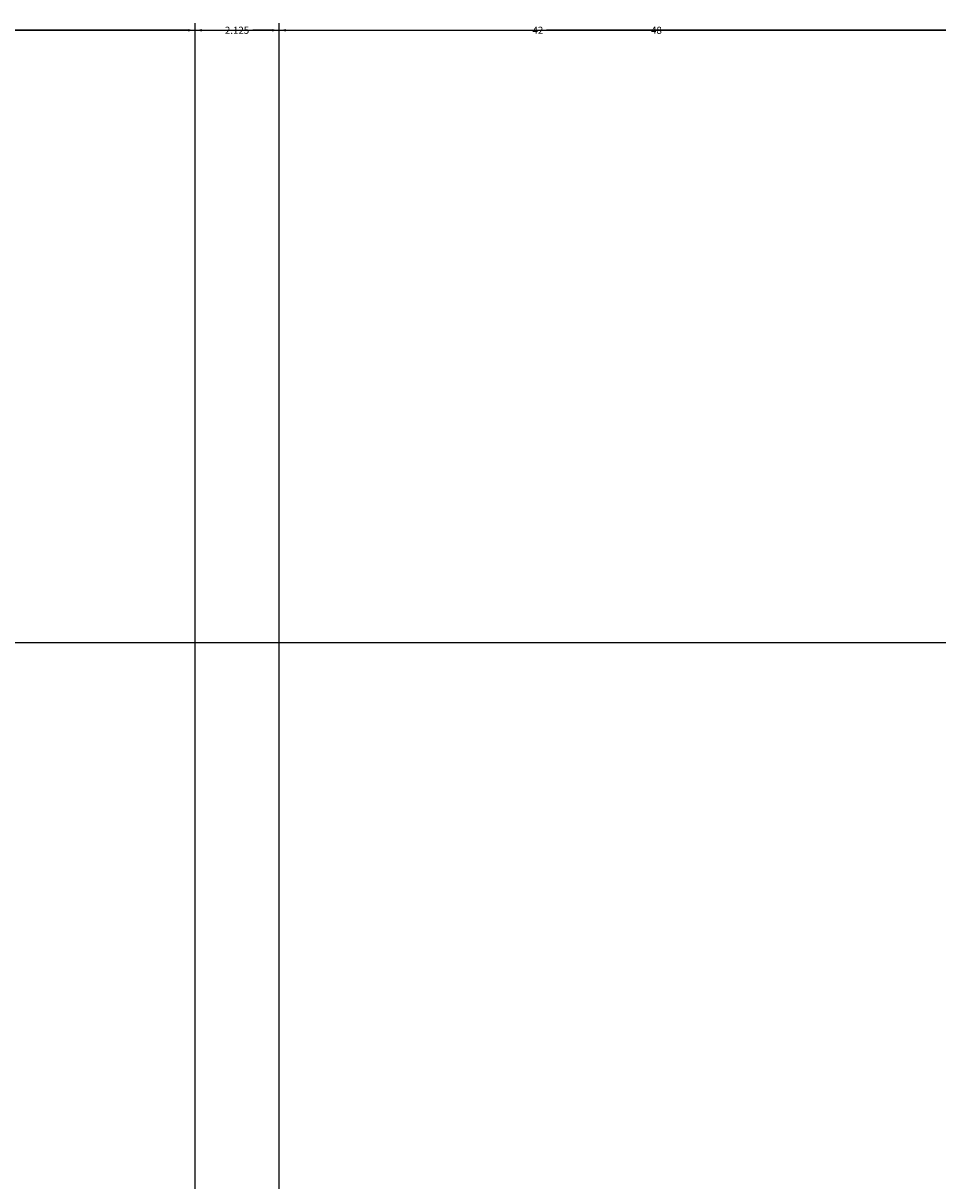
# Model space of a CAD drawing. Units: inches. Extents: x -6 to 289, y -8 to 323.
# Tile 102 of 107: x 196 to 219, y 294 to 323. Entities that reach past the tile are written whole.
import ezdxf

# ---------------------------------------------------------------- set-up
doc = ezdxf.new("R2010")
doc.units = ezdxf.units.IN
doc.header["$MEASUREMENT"] = 0
doc.layers.add('A-ANNO-DIMS', color=2, linetype='Continuous', lineweight=18)
doc.styles.get("Standard").update_dxf_attribs({"font": 'arial.ttf'})
doc.dimstyles.get("Standard").update_dxf_attribs({"dimtxt": 0.18, "dimasz": 0.18, "dimexe": 0.18, "dimexo": 0.0625, "dimgap": 0.09, "dimtad": 0, "dimtih": 1, "dimtoh": 1, "dimdec": 4, "dimzin": 0, "dimdsep": 46, "dimtxsty": 'Standard', "dimcen": 0.09, "dimadec": 0, "dimazin": 0, "dimtfac": 1, "dimtdec": 4, "dimtofl": 0, "dimtmove": 0, "dimatfit": 3, "dimfxl": 1, "dimtolj": 1, "dimtzin": 0, "dimarcsym": 0})

# ---------------------------------------------------------------- blocks, each defined once
blk = doc.blocks.new('*D13')
at = {"layer": 'A-ANNO-DIMS', "color": 0, "lineweight": -2, "transparency": 16777216}
for p, q in [((188.292, 226.951), (188.292, 322.969)), ((236.292, 226.951), (236.292, 322.969)), ((188.472, 322.789), (212.069, 322.789)), ((236.112, 322.789), (212.515, 322.789))]:
    blk.add_line(p, q, dxfattribs=at)
at = {"layer": 'A-ANNO-DIMS', "color": 0, "transparency": 16777216}
for points in [[(188.472, 322.819), (188.472, 322.759), (188.292, 322.789)], [(236.112, 322.819), (236.112, 322.759), (236.292, 322.789)]]:
    blk.add_solid(points, dxfattribs=at)
at = {"layer": 'Defpoints', "color": 0, "transparency": 16777216}
for p in [(236.292, 322.789), (188.292, 226.889), (236.292, 226.889)]:
    blk.add_point(p, dxfattribs=at)
at = {"layer": 'A-ANNO-DIMS', "color": 0, "transparency": 16777216, "insert": (212.292, 322.789), "char_height": 0.18, "attachment_point": 5}
blk.add_mtext('\\A1;48', dxfattribs=at)
blk = doc.blocks.new('*D27')
at = {"layer": 'A-ANNO-DIMS', "color": 0, "lineweight": -2, "transparency": 16777216}
for p, q in [((19.226, 307.289), (288.653, 307.289)), ((288.473, 307.109), (288.473, 277.471)), ((288.473, 247.469), (288.473, 277.107)), ((247.226, 247.289), (288.653, 247.289))]:
    blk.add_line(p, q, dxfattribs=at)
at = {"layer": 'A-ANNO-DIMS', "color": 0, "transparency": 16777216}
for points in [[(288.443, 307.109), (288.503, 307.109), (288.473, 307.289)], [(288.443, 247.469), (288.503, 247.469), (288.473, 247.289)]]:
    blk.add_solid(points, dxfattribs=at)
at = {"layer": 'Defpoints', "color": 0, "transparency": 16777216}
for p in [(19.164, 307.289), (288.473, 307.289), (247.164, 247.289)]:
    blk.add_point(p, dxfattribs=at)
at = {"layer": 'A-ANNO-DIMS', "color": 0, "transparency": 16777216, "insert": (288.473, 277.289), "char_height": 0.18, "attachment_point": 5}
blk.add_mtext('\\A1;60', dxfattribs=at)
blk = doc.blocks.new('*D80')
at = {"layer": 'A-ANNO-DIMS', "color": 0, "lineweight": -2, "transparency": 16777216}
for p, q in [((188.292, 116.842), (188.292, 322.969)), ((230.292, 116.842), (230.292, 322.969)), ((188.472, 322.789), (209.07, 322.789)), ((230.112, 322.789), (209.513, 322.789))]:
    blk.add_line(p, q, dxfattribs=at)
at = {"layer": 'A-ANNO-DIMS', "color": 0, "transparency": 16777216}
for points in [[(188.472, 322.819), (188.472, 322.759), (188.292, 322.789)], [(230.112, 322.819), (230.112, 322.759), (230.292, 322.789)]]:
    blk.add_solid(points, dxfattribs=at)
at = {"layer": 'Defpoints', "color": 0, "transparency": 16777216}
for p in [(230.292, 322.789), (188.292, 116.779), (230.292, 116.779)]:
    blk.add_point(p, dxfattribs=at)
at = {"layer": 'A-ANNO-DIMS', "color": 0, "transparency": 16777216, "insert": (209.292, 322.789), "char_height": 0.18, "attachment_point": 5}
blk.add_mtext('\\A1;42', dxfattribs=at)
blk = doc.blocks.new('*D96')
at = {"layer": 'A-ANNO-DIMS', "color": 0, "lineweight": -2, "transparency": 16777216}
for p, q in [((164.004, 159.411), (164.004, 322.969)), ((200.616, 159.411), (200.616, 322.969)), ((164.184, 322.789), (181.934, 322.789)), ((200.436, 322.789), (182.686, 322.789))]:
    blk.add_line(p, q, dxfattribs=at)
at = {"layer": 'A-ANNO-DIMS', "color": 0, "transparency": 16777216}
for points in [[(164.184, 322.819), (164.184, 322.759), (164.004, 322.789)], [(200.436, 322.819), (200.436, 322.759), (200.616, 322.789)]]:
    blk.add_solid(points, dxfattribs=at)
at = {"layer": 'Defpoints', "color": 0, "transparency": 16777216}
for p in [(200.616, 322.789), (164.004, 159.348), (200.616, 159.348)]:
    blk.add_point(p, dxfattribs=at)
at = {"layer": 'A-ANNO-DIMS', "color": 0, "transparency": 16777216, "insert": (182.31, 322.789), "char_height": 0.18, "attachment_point": 5}
blk.add_mtext('\\A1;36.61', dxfattribs=at)
blk = doc.blocks.new('*D97')
at = {"layer": 'A-ANNO-DIMS', "color": 0, "lineweight": -2, "transparency": 16777216}
for p, q in [((200.616, 159.411), (200.616, 322.969)), ((202.741, 159.411), (202.741, 322.969)), ((200.796, 322.789), (201.283, 322.789)), ((202.561, 322.789), (202.075, 322.789))]:
    blk.add_line(p, q, dxfattribs=at)
at = {"layer": 'A-ANNO-DIMS', "color": 0, "transparency": 16777216}
for points in [[(200.796, 322.819), (200.796, 322.759), (200.616, 322.789)], [(202.561, 322.819), (202.561, 322.759), (202.741, 322.789)]]:
    blk.add_solid(points, dxfattribs=at)
at = {"layer": 'Defpoints', "color": 0, "transparency": 16777216}
for p in [(202.741, 322.789), (200.616, 159.348), (202.741, 159.348)]:
    blk.add_point(p, dxfattribs=at)
at = {"layer": 'A-ANNO-DIMS', "color": 0, "transparency": 16777216, "insert": (201.679, 322.789), "char_height": 0.18, "attachment_point": 5}
blk.add_mtext('\\A1;2.125', dxfattribs=at)
blk = doc.blocks.new('*D98')
at = {"layer": 'A-ANNO-DIMS', "color": 0, "lineweight": -2, "transparency": 16777216}
for p, q in [((202.741, 159.411), (202.741, 322.969)), ((244.164, 159.411), (244.164, 322.969)), ((202.921, 322.789), (223.056, 322.789)), ((243.984, 322.789), (223.849, 322.789))]:
    blk.add_line(p, q, dxfattribs=at)
at = {"layer": 'A-ANNO-DIMS', "color": 0, "transparency": 16777216}
for points in [[(202.921, 322.819), (202.921, 322.759), (202.741, 322.789)], [(243.984, 322.819), (243.984, 322.759), (244.164, 322.789)]]:
    blk.add_solid(points, dxfattribs=at)
at = {"layer": 'Defpoints', "color": 0, "transparency": 16777216}
for p in [(244.164, 322.789), (202.741, 159.348), (244.164, 159.348)]:
    blk.add_point(p, dxfattribs=at)
at = {"layer": 'A-ANNO-DIMS', "color": 0, "transparency": 16777216, "insert": (223.452, 322.789), "char_height": 0.18, "attachment_point": 5}
blk.add_mtext('\\A1;41.42', dxfattribs=at)
blk = doc.blocks.new('*D108')
at = {"layer": 'A-ANNO-DIMS', "color": 0, "lineweight": -2, "transparency": 16777216}
for p, q in [((186.984, 291.541), (186.984, 322.969)), ((255.804, 291.541), (255.804, 322.969)), ((187.164, 322.789), (221, 322.789)), ((255.624, 322.789), (221.787, 322.789))]:
    blk.add_line(p, q, dxfattribs=at)
at = {"layer": 'A-ANNO-DIMS', "color": 0, "transparency": 16777216}
for points in [[(187.164, 322.819), (187.164, 322.759), (186.984, 322.789)], [(255.624, 322.819), (255.624, 322.759), (255.804, 322.789)]]:
    blk.add_solid(points, dxfattribs=at)
at = {"layer": 'Defpoints', "color": 0, "transparency": 16777216}
for p in [(255.804, 322.789), (186.984, 291.478), (255.804, 291.478)]:
    blk.add_point(p, dxfattribs=at)
at = {"layer": 'A-ANNO-DIMS', "color": 0, "transparency": 16777216, "insert": (221.394, 322.789), "char_height": 0.18, "attachment_point": 5}
blk.add_mtext('\\A1;68.82', dxfattribs=at)
blk = doc.blocks.new('*D118')
at = {"layer": 'A-ANNO-DIMS', "color": 0, "lineweight": -2, "transparency": 16777216}
for p, q in [((118.226, 307.289), (288.653, 307.289)), ((288.473, 307.109), (288.473, 300.659)), ((288.473, 293.846), (288.473, 300.295)), ((257.703, 293.666), (288.653, 293.666))]:
    blk.add_line(p, q, dxfattribs=at)
at = {"layer": 'A-ANNO-DIMS', "color": 0, "transparency": 16777216}
for points in [[(288.443, 307.109), (288.503, 307.109), (288.473, 307.289)], [(288.443, 293.846), (288.503, 293.846), (288.473, 293.666)]]:
    blk.add_solid(points, dxfattribs=at)
at = {"layer": 'Defpoints', "color": 0, "transparency": 16777216}
for p in [(118.164, 307.289), (288.473, 307.289), (257.641, 293.666)]:
    blk.add_point(p, dxfattribs=at)
at = {"layer": 'A-ANNO-DIMS', "color": 0, "transparency": 16777216, "insert": (288.473, 300.477), "char_height": 0.18, "attachment_point": 5}
blk.add_mtext('\\A1;13.623', dxfattribs=at)

msp = doc.modelspace()

# ---------------------------------------------------------------- dimensions: what is measured, and where the dimension line sits
at = {"layer": 'A-ANNO-DIMS'}
for base, p1, p2, override, picture, middle in [((200.6162, 322.7888), (164.0039, 159.3484), (200.6162, 159.3484), {"dimdec": 2, "dimlfac": 1, "dimrnd": 0, "dimzin": 0, "dimdsep": 46, "dimlunit": 2}, '*D96', (182.3101, 322.7888)), ((255.8036, 322.7888), (186.9837, 291.4781), (255.8036, 291.4781), {"dimdec": 2, "dimlfac": 1, "dimrnd": 0, "dimzin": 0, "dimdsep": 46, "dimlunit": 2}, '*D108', (221.3936, 322.7888)), ((236.2918, 322.7888), (188.2918, 226.8887), (236.2918, 226.8887), {"dimdec": 0, "dimlfac": 1, "dimrnd": 0, "dimzin": 0, "dimdsep": 46, "dimlunit": 2}, '*D13', (212.2918, 322.7888)), ((230.2918, 322.7888), (188.2918, 116.7795), (230.2918, 116.7795), {"dimdec": 0, "dimlfac": 1, "dimrnd": 0, "dimzin": 0, "dimdsep": 46, "dimlunit": 2}, '*D80', (209.2918, 322.7888)), ((202.741, 322.7888), (200.6162, 159.3484), (202.741, 159.3484), {"dimdec": 3, "dimlfac": 1, "dimrnd": 0, "dimzin": 0, "dimdsep": 46, "dimlunit": 2}, '*D97', (201.6786, 322.7888)), ((244.1638, 322.7888), (202.741, 159.3484), (244.1638, 159.3484), {"dimdec": 2, "dimlfac": 1, "dimrnd": 0, "dimzin": 0, "dimdsep": 46, "dimlunit": 2}, '*D98', (223.4524, 322.7888))]:
    dim = msp.add_linear_dim(base=base, p1=p1, p2=p2, dimstyle='Standard', override=override, dxfattribs=at)
    dim.commit()
    dim.dimension.update_dxf_attribs({"geometry": picture, "text_midpoint": middle})
for p1, p2, override, picture, middle in [((247.1638, 247.2888), (19.1638, 307.2888), {"dimdec": 0, "dimlfac": 1, "dimrnd": 0, "dimzin": 0, "dimdsep": 46, "dimlunit": 2}, '*D27', (288.4733, 277.2888)), ((257.6407, 293.6657), (118.1638, 307.2888), {"dimdec": 3, "dimlfac": 1, "dimrnd": 0, "dimzin": 0, "dimdsep": 46, "dimlunit": 2}, '*D118', (288.4733, 300.4773))]:
    dim = msp.add_linear_dim(base=(288.4733, 307.2888), p1=p1, p2=p2, angle=90, dimstyle='Standard', override=override, dxfattribs=at)
    dim.commit()
    dim.dimension.update_dxf_attribs({"geometry": picture, "text_midpoint": middle})

doc.saveas('drawing.dxf')
